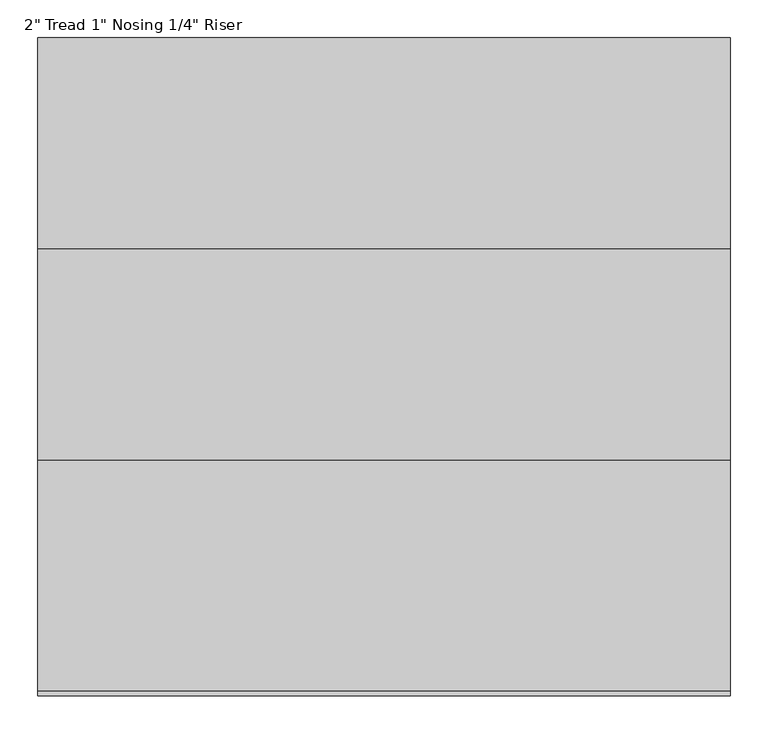
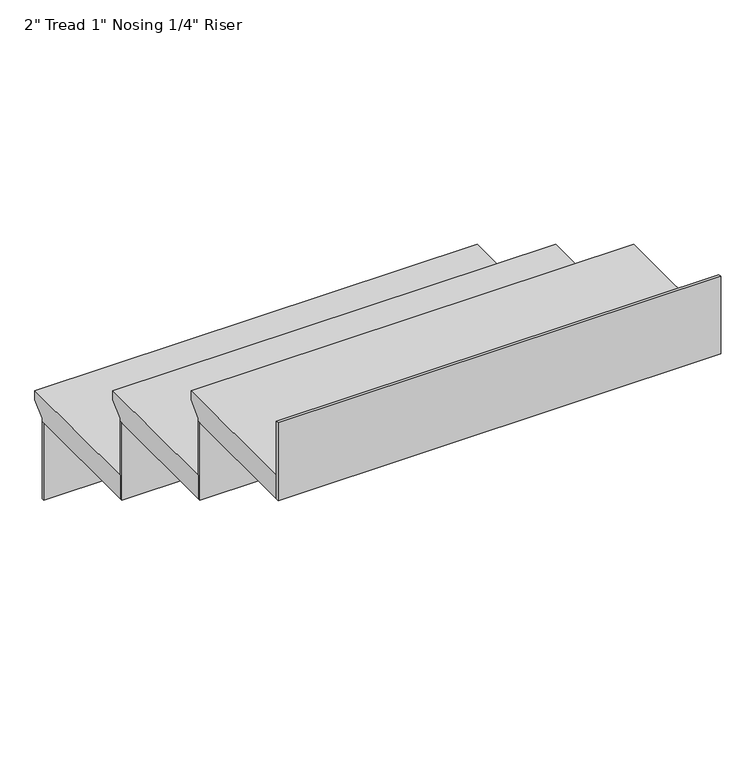
"""IFC4 building model written with IfcOpenShell, lengths in millimetres: stair flight geometry."""

from ifc_helpers import new_model, si_unit, frame, origin, place, context, project, spatial, polyline, outline, extrude, source, transform, mapped, element, save


def stair_flight_c8914c85(model_context):
    return source(origin(), model_context, "Body", "SweptSolid", [
        extrude(outline(polyline([(-19826.9851539, 46062.6172466), (-19522.1851539, 46062.6172466), (-19522.1851539, 46043.5672466), (-19547.5851539, 46018.1672466), (-19547.5851539, 46011.8172466), (-19826.9851539, 46011.8172466), (-19826.9851539, 46062.6172466)])), frame((-2296.6415084, 0.0, 0.0), z_axis=(1.0, 0.0, 0.0), x_axis=(0.0, 1.0, 0.0)), (0.0, 0.0, 1.0), 914.4),
        extrude(outline(polyline([(-2296.6415084, -19553.9351539), (-2296.6415084, -19547.5851539), (-1382.2415084, -19547.5851539), (-1382.2415084, -19553.9351539), (-2296.6415084, -19553.9351539)])), frame((0.0, 0.0, 45842.4839133), z_axis=(0.0, 0.0, 1.0), x_axis=(1.0, 0.0, 0.0)), (0.0, 0.0, 1.0), 169.3333333),
        extrude(outline(polyline([(-2296.6415084, -19833.3351539), (-2296.6415084, -19826.9851539), (-1382.2415084, -19826.9851539), (-1382.2415084, -19833.3351539), (-2296.6415084, -19833.3351539)])), frame((0.0, 0.0, 46011.8172466), z_axis=(0.0, 0.0, 1.0), x_axis=(1.0, 0.0, 0.0)), (0.0, 0.0, 1.0), 169.3333333),
        extrude(outline(polyline([(-20106.3851539, 46231.9505799), (-19801.5851539, 46231.9505799), (-19801.5851539, 46212.9005799), (-19826.9851539, 46187.5005799), (-19826.9851539, 46181.1505799), (-20106.3851539, 46181.1505799), (-20106.3851539, 46231.9505799)])), frame((-2296.6415084, 0.0, 0.0), z_axis=(1.0, 0.0, 0.0), x_axis=(0.0, 1.0, 0.0)), (0.0, 0.0, 1.0), 914.4),
        extrude(outline(polyline([(-2296.6415084, -20112.7351539), (-2296.6415084, -20106.3851539), (-1382.2415084, -20106.3851539), (-1382.2415084, -20112.7351539), (-2296.6415084, -20112.7351539)])), frame((0.0, 0.0, 46181.1505799), z_axis=(0.0, 0.0, 1.0), x_axis=(1.0, 0.0, 0.0)), (0.0, 0.0, 1.0), 169.3333333),
        extrude(outline(polyline([(-2296.6415084, -20392.1351539), (-2296.6415084, -20385.7851539), (-1382.2415084, -20385.7851539), (-1382.2415084, -20392.1351539), (-2296.6415084, -20392.1351539)])), frame((0.0, 0.0, 46350.4839133), z_axis=(0.0, 0.0, 1.0), x_axis=(1.0, 0.0, 0.0)), (0.0, 0.0, 1.0), 169.3333333),
        extrude(outline(polyline([(-20385.7851539, 46401.2839133), (-20080.9851539, 46401.2839133), (-20080.9851539, 46382.2339133), (-20106.3851539, 46356.8339133), (-20106.3851539, 46350.4839133), (-20385.7851539, 46350.4839133), (-20385.7851539, 46401.2839133)])), frame((-2296.6415084, 0.0, 0.0), z_axis=(1.0, 0.0, 0.0), x_axis=(0.0, 1.0, 0.0)), (0.0, 0.0, 1.0), 914.4),
    ])


if __name__ == "__main__":
    model = new_model("IFC4")
    model_context = context("Model", 3, world=origin())
    ifc_project = project(units=[si_unit("LENGTHUNIT", "METRE", prefix="MILLI")], contexts=[model_context])
    site = spatial("IfcSite", under=ifc_project)
    building = spatial("IfcBuilding", under=site)
    placement = place(None, origin())
    stair_flight_shape = stair_flight_c8914c85(model_context)
    element("IfcStairFlight", 1, ObjectType="2\" Tread 1\" Nosing 1/4\" Riser", at=placement, inside=building, context=model_context, shape_type="MappedRepresentation", body=[
        mapped(stair_flight_shape, transform((0.0, 0.0, 0.0), x_axis=(1.0, 0.0, 0.0), y_axis=(0.0, 1.0, 0.0), z_axis=(0.0, 0.0, 1.0))),
    ])
    save(model, "model.ifc")
